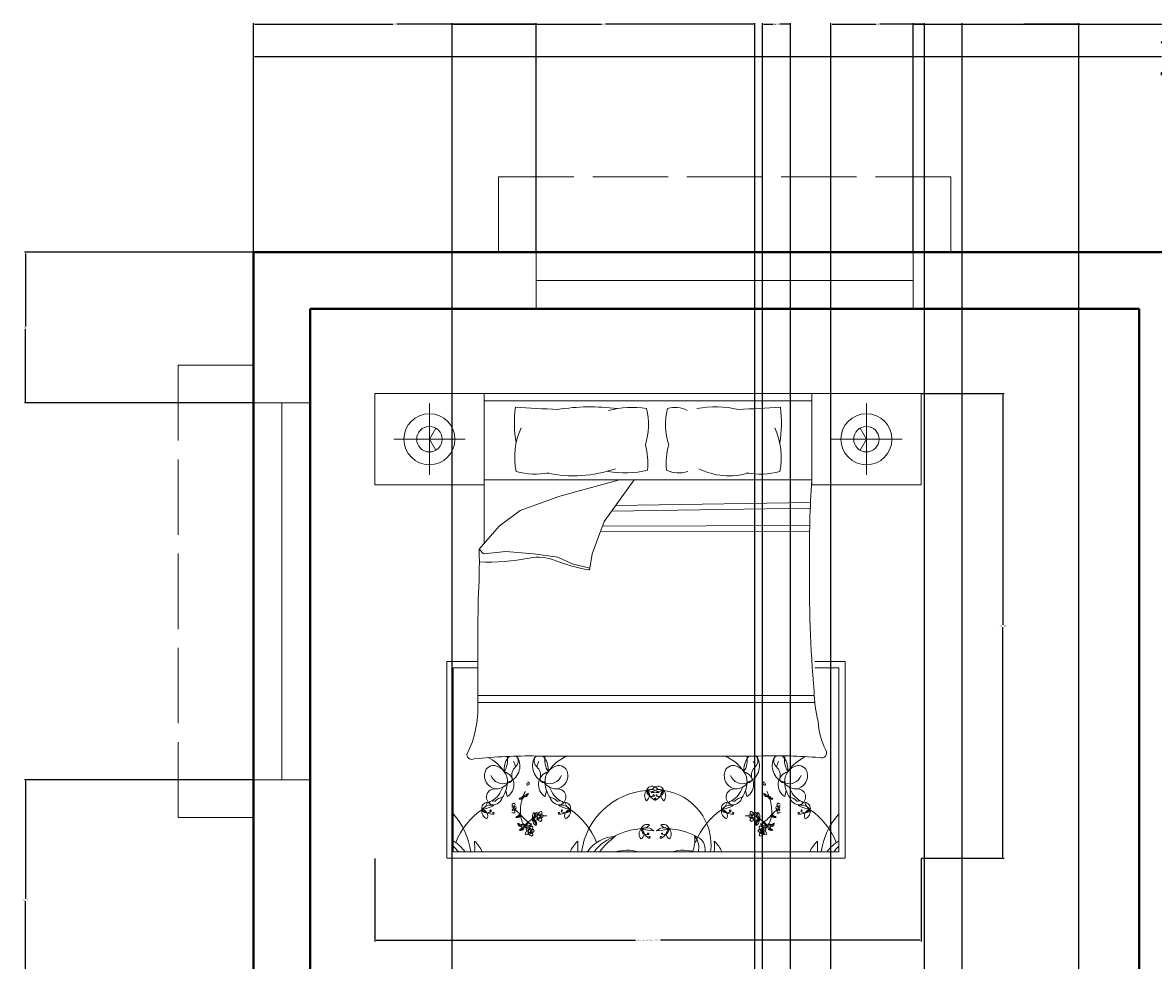
# Model space of a CAD drawing. Units: inches. Extents: x -22 to 362, y -469 to 42.
# Tile 5 of 6: x -22 to 158, y -107 to 42. Entities that reach past the tile are written whole.
import ezdxf

# ---------------------------------------------------------------- set-up
doc = ezdxf.new("R2010")
doc.units = ezdxf.units.IN
doc.header["$MEASUREMENT"] = 0
doc.linetypes.add('ACAD_ISO02W100', pattern=[15, 12, -3])
for name, color, linetype, lineweight in [('A-ANNO-DIMS', 2, 'Continuous', 18), ('A-FURN', 8, 'Continuous', 18), ('A-GLAZ', 4, 'Continuous', 20), ('A-ROOF-OVHD', 8, 'ACAD_ISO02W100', 18), ('A-WALL', 7, 'Continuous', 40)]:
    doc.layers.add(name, color=color, linetype=linetype, lineweight=lineweight)
doc.styles.get("Standard").update_dxf_attribs({"font": 'arial.ttf'})
doc.dimstyles.get("Standard").update_dxf_attribs({"dimtxt": 0.18, "dimasz": 0.18, "dimexe": 0.18, "dimexo": 0.0625, "dimgap": 0.09, "dimtad": 0, "dimtih": 1, "dimtoh": 1, "dimdec": 0, "dimzin": 0, "dimdsep": 46, "dimlunit": 3, "dimtxsty": 'Standard', "dimcen": 0.09, "dimadec": 0, "dimazin": 0, "dimtfac": 1, "dimtdec": 0, "dimtofl": 0, "dimtmove": 0, "dimatfit": 3, "dimfxl": 1, "dimtolj": 1, "dimtzin": 0, "dimarcsym": 0})

# ---------------------------------------------------------------- blocks, each defined once
blk = doc.blocks.new('*D5')
at = {"layer": 'A-ANNO-DIMS', "color": 0, "lineweight": -2, "transparency": 16777216}
for p, q in [((15.01, 5.76), (15.01, 37.04)), ((15.19, 36.86), (159.53, 36.86)), ((314.33, 36.86), (169.99, 36.86)), ((314.51, 5.76), (314.51, 37.04))]:
    blk.add_line(p, q, dxfattribs=at)
at = {"layer": 'A-ANNO-DIMS', "color": 0, "transparency": 16777216}
for points in [[(15.19, 36.89), (15.19, 36.83), (15.01, 36.86)], [(314.33, 36.89), (314.33, 36.83), (314.51, 36.86)]]:
    blk.add_solid(points, dxfattribs=at)
at = {"layer": 'Defpoints', "color": 0, "transparency": 16777216}
for p in [(314.51, 36.86), (15.01, 5.69), (314.51, 5.69)]:
    blk.add_point(p, dxfattribs=at)
at = {"layer": 'A-ANNO-DIMS', "color": 0, "transparency": 16777216, "insert": (164.76, 36.86), "char_height": 6, "attachment_point": 5}
blk.add_mtext("\\A1;25'", dxfattribs=at)
blk = doc.blocks.new('WIN-60-WALL9')
for p, q in [((0, 9), (60, 9)), ((0, 0), (0, 9)), ((60, 9), (60, 0)), ((0, 4.5), (60, 4.5)), ((60, 0), (0, 0))]:
    blk.add_line(p, q)
blk = doc.blocks.new('WINDOW-SHADE-72')
for p, q in [((12, 72), (0, 72)), ((12, 0), (12, 72)), ((0, 0), (12, 0))]:
    blk.add_line(p, q)
blk = doc.blocks.new('BED-DOUBLE-WITH-NIGHTSTANDS')
for p, q in [((0, 73.94), (86.94, 73.94)), ((17.39, 73.94), (17.39, 50.07)), ((8.69, 61.01), (8.69, 72.37)), ((69.55, 72.82), (17.39, 72.82)), ((78.25, 61.01), (78.25, 72.37)), ((14.37, 66.69), (3.01, 66.69)), ((72.57, 66.69), (83.93, 66.69)), ((17.39, 60.2), (69.55, 60.2)), ((29.46, 57.61), (38.94, 60.2)), ((41.27, 60.2), (36.51, 53.57)), ((23.13, 55.33), (29.46, 57.61)), ((69.32, 56.59), (38.37, 56.15)), ((19.78, 52.86), (23.13, 55.33)), ((69.29, 55.69), (37.72, 55.25)), ((16.61, 49.17), (19.78, 52.86)), ((36.51, 53.57), (34.57, 48.46)), ((69.24, 52.96), (36.23, 52.83)), ((69.24, 52.06), (35.89, 51.93)), ((17.31, 48.46), (16.61, 49.17)), ((20.84, 48.81), (17.31, 48.46)), ((25.24, 48.46), (20.84, 48.81)), ((29.11, 47.94), (25.24, 48.46)), ((31.4, 46.88), (29.11, 47.94)), ((34.22, 46.18), (31.4, 46.88)), ((34.57, 48.46), (34.22, 46.18)), ((11.48, 31.32), (16.39, 31.32)), ((11.48, 0), (11.48, 31.32)), ((70.04, 31.32), (74.86, 31.32)), ((74.86, 31.32), (74.86, 0)), ((16.39, 30.31), (12.48, 30.31)), ((12.48, 30.31), (12.48, 1.01)), ((73.85, 30.31), (70.02, 30.31)), ((73.85, 1.01), (73.85, 30.31)), ((69.95, 25.9), (16.39, 25.9)), ((70.03, 24.81), (16.39, 24.81)), ((61.12, 16.27), (25.82, 16.27)), ((21.05, 9.82), (20.86, 10.8)), ((27.13, 9.82), (27.32, 10.8)), ((59.21, 9.82), (59.02, 10.8)), ((65.28, 9.82), (65.48, 10.8)), ((74.86, 0), (11.48, 0)), ((12.48, 1.01), (73.85, 1.01))]:
    blk.add_line(p, q)
for points in [[(17.39, 59.45), (0, 59.45), (0, 73.94)], [(69.55, 73.94), (69.55, 59.45), (86.94, 59.45), (86.94, 73.94)], [(8.69, 66.69), (9.71, 68.45)], [(78.25, 66.69), (77.23, 68.45)], [(8.69, 66.69), (9.71, 64.94)], [(78.25, 66.69), (77.23, 64.94)]]:
    blk.add_lwpolyline(points)
for points in [[(22.38, 71.77, 0.074897), (22.49, 66.09, -0.472817)], [(43.06, 65.77, 0.14099), (43.24, 71.57, 0.235245)], [(46.78, 65.77, -0.14099), (46.6, 71.57, -0.235245)], [(64.56, 71.77, -0.074897), (64.45, 66.09, 0.472817)], [(16.43, 41.21, 0.001242), (16.39, 24.71, -0.127202), (14.64, 16.49)], [(69.92, 26.58, 0.056112), (70.55, 21.8, 0.095341), (71.78, 17.19)]]:
    blk.add_lwpolyline(points, format="xyb")
for centre, radius in [((8.69, 66.69), 4.06), ((78.25, 66.69), 4.06), ((8.69, 66.69), 2.03), ((78.25, 66.69), 2.03), ((26.07, 6.67), 0.221), ((60.26, 6.67), 0.221), ((24.62, 4.34), 0.221), ((61.71, 4.34), 0.221)]:
    blk.add_circle(centre, radius)
for centre, radius, start, end in [((70.3, 899.16), 828.77, 266.68521, 267.14978), ((34.29, 40.31), 31.53, 82.2196, 99.497), ((40.95, 56.24), 15.49, 81.5249, 103.96), ((47.79, 67.44), 4.3, 63.3437, 106.1026), ((54.24, 56.56), 15.28, 76.3427, 101.1841), ((16.64, 899.16), 828.77, 272.85022, 273.31479), ((33.46, 63.81), 11.21, 155.1316, 191.7583), ((53.48, 63.81), 11.21, 348.2417, 24.8684), ((32.81, 62.87), 10.65, 354.0129, 15.8293), ((57.02, 62.87), 10.65, 164.1707, 185.9871), ((25.48, 72.79), 11.65, 255.1039, 281.0369), ((31.62, 81.07), 20.21, 258.0397, 289.2615), ((39.8, 76.66), 15.33, 259.8617, 283.6238), ((48.38, 65.93), 4.61, 245.0183, 288.5407), ((56.43, 71.93), 11.07, 243.8761, 286.1746), ((61.46, 72.79), 11.65, 258.9631, 284.8961), ((225.41, 49.57), 156.22, 176.1, 180.9282), ((-63.11, 47.01), 79.74, 355.8294, 1.553), ((18.1, 79.95), 32.81, 267.4519, 281.3392), ((25.94, 40.84), 7.08, 66.2616, 101.3392), ((40.26, 79.03), 33.72, 250.1194, 259.3383), ((272.96, 43.89), 203.78, 179.1145, 184.8735), ((34.02, 46.1), 0.21, 268.8623, 19.7536), ((15.44, 16.54), 0.802, 183.98, 297.3412), ((24.78, -74.23), 90.51, 89.3433, 95.6887), ((17.52, 15.63), 3.6, 328.8218, 9.1554), ((21.98, 15.31), 1.05, 120.0293, 142.325), ((21.98, 15.31), 1.05, 44.4517, 63.558), ((26.2, 15.31), 1.05, 113.229, 135.5483), ((26.2, 15.31), 1.05, 37.675, 66.7144), ((30.66, 15.63), 3.6, 169.7133, 211.1782), ((33.07, 10.15), 6.58, 111.4941, 146.3329), ((53.26, 10.15), 6.58, 33.6671, 68.5059), ((55.68, 15.63), 3.6, 328.8218, 10.2867), ((60.14, 15.31), 1.05, 113.2856, 142.325), ((60.14, 15.31), 1.05, 44.4517, 66.7144), ((63.78, -68.29), 84.6, 85.2402, 91.8035), ((64.35, 15.31), 1.05, 106.6343, 135.5483), ((64.35, 15.31), 1.05, 37.675, 72.5814), ((68.82, 15.63), 3.6, 169.249, 211.1782), ((71.12, 16.75), 0.792, 246.5219, 33.8264), ((18.94, 13.31), 1.47, 84.4856, 181.0538), ((15.1, 10.15), 6.58, 33.6671, 63.2997), ((18.49, 12.22), 2.61, 355.2933, 76.921), ((23.92, 14.06), 3.35, 145.785, 184.7304), ((20.31, 14.69), 2.77, 289.2822, 29.1751), ((23.58, 13.21), 1.78, 131.5653, 195.1471), ((19.89, 14.19), 2.5, 7.436, 29.9149), ((21.54, 15.52), 1.3, 311.5653, 23.8354), ((27.87, 14.69), 2.77, 150.8249, 250.7178), ((26.64, 15.52), 1.3, 156.1646, 228.4347), ((24.59, 13.21), 1.78, 344.8529, 48.4347), ((28.29, 14.19), 2.5, 150.0851, 172.564), ((24.25, 14.06), 3.35, 355.2696, 34.215), ((29.69, 12.22), 2.61, 103.079, 184.7067), ((29.24, 13.31), 1.47, 358.9462, 95.5144), ((57.09, 13.31), 1.47, 84.4856, 181.0538), ((56.64, 12.22), 2.61, 355.2933, 76.921), ((62.08, 14.06), 3.35, 145.785, 184.7304), ((58.46, 14.69), 2.77, 289.2822, 29.1751), ((61.74, 13.21), 1.78, 131.5653, 195.1471), ((58.05, 14.19), 2.5, 7.436, 29.9149), ((59.69, 15.52), 1.3, 311.5653, 23.8354), ((66.03, 14.69), 2.77, 150.8249, 250.7178), ((64.8, 15.52), 1.3, 156.1646, 228.4347), ((62.75, 13.21), 1.78, 344.8529, 48.4347), ((66.44, 14.19), 2.5, 150.0851, 172.564), ((62.41, 14.06), 3.35, 355.2696, 34.215), ((67.85, 12.22), 2.61, 103.079, 184.7067), ((71.23, 10.15), 6.58, 113.6453, 146.3329), ((67.4, 13.31), 1.47, 358.9462, 95.5144), ((19.54, 13.1), 2.08, 174.9449, 262.8857), ((20.36, 13.89), 2.02, 201.5819, 291.4221), ((19.97, 11.7), 2.16, 299.9085, 73.1337), ((21.34, 12.6), 0.54, 257.3041, 15.1471), ((28.2, 11.7), 2.16, 106.8663, 240.0915), ((26.84, 12.6), 0.54, 164.8529, 282.6959), ((27.82, 13.89), 2.02, 248.5779, 338.4181), ((28.64, 13.1), 2.08, 277.1143, 5.0551), ((57.7, 13.1), 2.08, 174.9449, 262.8857), ((58.51, 13.89), 2.02, 201.5819, 291.4221), ((58.13, 11.7), 2.16, 299.9085, 73.1337), ((59.5, 12.6), 0.54, 257.3041, 15.1471), ((66.36, 11.7), 2.16, 106.8663, 240.0915), ((64.99, 12.6), 0.54, 164.8529, 282.6959), ((65.98, 13.89), 2.02, 248.5779, 338.4181), ((66.79, 13.1), 2.08, 277.1143, 5.0551), ((19.06, 9.75), 1.3, 80.264, 250.8688), ((16.47, 12.62), 4.1, 301.2614, 341.7045), ((19.18, 13.56), 2.53, 272.3591, 324.0401), ((16.44, 12.29), 4.67, 326.2883, 356.5076), ((23.92, 14.06), 3.35, 212.7011, 216.3445), ((24.34, 11.79), 0.168, 102.7051, 280.4384), ((24.32, 11.89), 0.272, 280.4384, 100.4136), ((24.25, 14.06), 3.35, 323.6555, 327.2989), ((29, 13.56), 2.53, 215.9599, 267.6409), ((31.74, 12.29), 4.67, 183.4924, 213.7117), ((31.7, 12.62), 4.1, 198.2955, 238.7386), ((29.12, 9.75), 1.3, 289.1312, 99.736), ((44.17, 10.53), 0.941, 63.0274, 163.8037), ((43.21, 12.73), 1.94, 271.4585, 315.3727), ((44, 9.16), 1.79, 45.5411, 114.3101), ((45.23, 9.16), 1.79, 65.6899, 134.4589), ((45.07, 10.53), 0.941, 16.1963, 116.9726), ((46.02, 12.73), 1.94, 224.6273, 268.5415), ((57.22, 9.75), 1.3, 80.264, 250.8688), ((54.63, 12.62), 4.1, 301.2614, 341.7045), ((57.34, 13.56), 2.53, 272.3591, 324.0401), ((54.59, 12.29), 4.67, 326.2883, 356.5076), ((62.08, 14.06), 3.35, 212.7011, 216.3445), ((62.01, 11.89), 0.272, 79.5864, 259.5616), ((62, 11.79), 0.168, 259.5616, 77.2949), ((62.41, 14.06), 3.35, 323.6555, 327.2989), ((67.16, 13.56), 2.53, 215.9599, 267.6409), ((69.9, 12.29), 4.67, 183.4924, 213.7117), ((69.86, 12.62), 4.1, 198.2955, 238.7386), ((67.27, 9.75), 1.3, 289.1312, 99.736), ((18.79, 8.34), 0.8, 63.9755, 143.2681), ((18.75, 10.14), 1.63, 265.969, 344.3045), ((20.5, 7.98), 1.74, 96.1662, 141.5825), ((23.38, 9.2), 0.456, 101.3256, 154.4621), ((22.72, 10.74), 1.37, 280.2588, 300.656), ((23.04, 11.84), 2.45, 268.3264, 277.1302), ((30.36, 7.41), 7.2, 163.5842, 183.8277), ((22.42, 10.74), 1.4, 308.2101, 316.3071), ((23.28, 9.82), 0.417, 278.3432, 4.2869), ((23.05, 10.19), 0.729, 300.656, 332.6341), ((23.6, 9.71), 0.177, 55.7657, 157.4417), ((30.36, 7.41), 7.2, 153.0032, 159.8941), ((23.87, 9.87), 0.177, 84.3784, 186.0543), ((23.71, 10.58), 0.729, 269.1859, 301.164), ((23.92, 10.21), 0.417, 237.5332, 323.4768), ((23.52, 11.4), 1.4, 285.5129, 293.6099), ((23.37, 11.14), 1.37, 301.164, 321.5612), ((24.43, 9.82), 0.456, 87.3579, 140.4944), ((22.26, 11.38), 2.45, 324.6898, 333.4936), ((27.67, 7.98), 1.74, 38.4175, 83.8338), ((29.43, 10.14), 1.63, 195.6955, 274.031), ((29.38, 8.34), 0.8, 36.7319, 116.0245), ((44.15, -0.52), 11.35, 94.4623, 172.255), ((44.2, 9.95), 1.26, 137.7873, 219.1145), ((42.77, 9.99), 0.948, 298.5391, 58.3627), ((45.64, 18.38), 7.94, 252.593, 267.2582), ((44.19, 10.76), 0.929, 177.7585, 283.852), ((45.98, 11.73), 2.87, 198.9159, 238.011), ((43.59, 18.38), 7.94, 272.7418, 287.407), ((44.38, 9.98), 0.123, 283.852, 219.9245), ((44.53, 9.41), 0.141, 238.011, 71.5592), ((44.56, 9.48), 0.0685, 71.5592, 188.0167), ((44.7, 9.41), 0.141, 108.4408, 301.989), ((44.68, 9.48), 0.0685, 351.9833, 108.4408), ((44.84, 10.03), 0.074, 320.1909, 256.0209), ((43.25, 11.73), 2.87, 301.989, 341.0841), ((45.04, 10.76), 0.929, 256.148, 2.2415), ((46.47, 9.99), 0.948, 121.6373, 241.4609), ((45.04, 9.95), 1.26, 320.8855, 42.2127), ((44.72, 2.1), 8.79, 352.8636, 81.8197), ((56.95, 8.34), 0.8, 63.9755, 143.2681), ((56.91, 10.14), 1.63, 265.969, 344.3045), ((58.66, 7.98), 1.74, 96.1662, 141.5825), ((62.96, 11.14), 1.37, 218.4388, 238.836), ((61.9, 9.82), 0.456, 39.5056, 92.6421), ((64.08, 11.38), 2.45, 206.5064, 215.3102), ((62.41, 10.21), 0.417, 216.5232, 302.4668), ((62.63, 10.58), 0.729, 238.836, 270.8141), ((62.82, 11.4), 1.4, 246.3901, 254.4871), ((55.97, 7.41), 7.2, 20.1059, 26.9968), ((62.46, 9.87), 0.177, 353.9457, 95.6216), ((62.74, 9.71), 0.177, 22.5583, 124.2343), ((63.05, 9.82), 0.417, 175.7131, 261.6568), ((63.28, 10.19), 0.729, 207.3659, 239.344), ((55.97, 7.41), 7.2, 356.1723, 16.4158), ((63.91, 10.74), 1.4, 223.6929, 231.7899), ((63.61, 10.74), 1.37, 239.344, 259.7412), ((63.3, 11.84), 2.45, 262.8698, 271.6736), ((62.96, 9.2), 0.456, 25.5379, 78.6744), ((67.59, 10.14), 1.63, 195.6955, 274.031), ((65.83, 7.98), 1.74, 38.4175, 83.8338), ((67.54, 8.34), 0.8, 36.7319, 116.0245), ((23.45, -1.64), 11.35, 124.3865, 158.5908), ((18.27, 7.46), 1.26, 167.7115, 249.0387), ((17.96, 7.95), 0.941, 92.9516, 193.728), ((16.03, 9.38), 1.94, 301.3827, 345.2969), ((18.5, 6.68), 1.79, 75.4653, 144.2343), ((15.32, 15.48), 7.94, 282.5173, 297.1824), ((17.01, 6.78), 0.948, 328.4633, 88.2869), ((18.93, 9.89), 2.87, 228.8402, 267.9352), ((17.86, 8.16), 0.929, 207.6827, 313.7762), ((18.42, 7.57), 0.123, 313.7762, 249.7183), ((18.82, 7.23), 0.0685, 101.4834, 217.9409), ((18.83, 7.16), 0.141, 267.9352, 101.4834), ((22.09, 8.33), 0.369, 101.5637, 142.6358), ((21.78, 7.99), 0.221, 273.2768, 86.7232), ((22.08, 7.58), 0.366, 217.7621, 259.0403), ((22.04, 8.2), 0.211, 91.1081, 181.8675), ((22.48, 8.06), 0.672, 203.4276, 227.6104), ((22.26, 7.77), 0.458, 80.3487, 133.6538), ((22.18, 8.15), 0.362, 229.7889, 317.6792), ((21.79, 8.62), 0.532, 288.7263, 352.5032), ((21.77, 7.38), 0.515, 355.053, 68.3618), ((22.18, 7.3), 0.725, 83.0852, 105.7171), ((22.15, 8.59), 0.171, 345.2356, 144.9248), ((22.12, 7.35), 0.17, 232.4737, 355.053), ((17.16, 1.28), 8.25, 43.1541, 52.0459), ((22.31, 8.03), 0.191, 317.6792, 80.3487), ((24.38, 7), 1.01, 304.5369, 16.3699), ((25.78, 6.72), 0.714, 127.3105, 187.9252), ((24.8, 6.8), 0.733, 355.0106, 41.658), ((25.83, 6.98), 0.302, 126.1046, 271.4281), ((25.8, 7.06), 0.217, 353.7526, 131.7054), ((26.38, 7.01), 0.369, 101.5637, 176.365), ((26.08, 7.3), 0.532, 288.7263, 352.5032), ((26.45, 7.28), 0.171, 345.2356, 144.9248), ((29.34, 7.16), 0.141, 78.5166, 272.0648), ((29.68, 6.68), 1.79, 35.7657, 104.5347), ((32.86, 15.48), 7.94, 242.8176, 257.4827), ((29.24, 9.89), 2.87, 272.0648, 311.1598), ((29.36, 7.23), 0.0685, 322.0591, 78.5166), ((30.31, 8.16), 0.929, 226.2238, 332.3173), ((29.77, 7.62), 0.074, 290.2667, 226.2271), ((31.16, 6.78), 0.948, 91.7131, 211.5367), ((30.22, 7.95), 0.941, 346.272, 87.0484), ((32.14, 9.38), 1.94, 194.7031, 238.6173), ((29.9, 7.46), 1.26, 290.9613, 12.2885), ((24.72, -1.64), 11.35, 21.4092, 55.6135), ((61.61, -1.64), 11.35, 124.3865, 158.5908), ((56.11, 7.95), 0.941, 92.9516, 193.728), ((56.43, 7.46), 1.26, 167.7115, 249.0387), ((54.19, 9.38), 1.94, 301.3827, 345.2969), ((56.66, 6.68), 1.79, 75.4653, 144.2343), ((53.48, 15.48), 7.94, 282.5173, 297.1824), ((56.02, 8.16), 0.929, 207.6827, 313.7762), ((57.09, 9.89), 2.87, 228.8402, 267.9352), ((55.17, 6.78), 0.948, 328.4633, 88.2869), ((56.58, 7.57), 0.123, 313.7762, 249.7183), ((56.98, 7.23), 0.0685, 101.4834, 217.9409), ((56.99, 7.16), 0.141, 267.9352, 101.4834), ((59.89, 7.28), 0.171, 35.0752, 194.7644), ((60.25, 7.3), 0.532, 187.4968, 251.2737), ((59.95, 7.01), 0.369, 3.635, 78.4363), ((60.54, 7.06), 0.217, 48.2946, 186.2474), ((60.51, 6.98), 0.302, 268.5719, 53.8954), ((61.54, 6.8), 0.733, 138.342, 184.9894), ((61.96, 7), 1.01, 163.6301, 235.4631), ((60.55, 6.72), 0.714, 352.0748, 52.6895), ((69.18, 1.28), 8.25, 127.9541, 136.8459), ((64.03, 8.03), 0.191, 99.6513, 222.3208), ((64.15, 8.15), 0.362, 222.3208, 310.2111), ((64.07, 7.77), 0.458, 46.3462, 99.6513), ((64.18, 8.59), 0.171, 35.0752, 194.7644), ((64.54, 8.62), 0.532, 187.4968, 251.2737), ((64.56, 7.38), 0.515, 111.6382, 184.947), ((64.22, 7.35), 0.17, 184.947, 307.5263), ((64.16, 7.3), 0.725, 74.2829, 96.9148), ((64.29, 8.2), 0.211, 358.1325, 88.8919), ((63.86, 8.06), 0.672, 312.3896, 336.5724), ((64.25, 8.33), 0.369, 37.3642, 78.4363), ((64.25, 7.58), 0.366, 280.9597, 322.2379), ((64.55, 7.99), 0.221, 93.2768, 266.7232), ((67.5, 7.16), 0.141, 78.5166, 272.0648), ((67.84, 6.68), 1.79, 35.7657, 104.5347), ((71.01, 15.48), 7.94, 242.8176, 257.4827), ((67.4, 9.89), 2.87, 272.0648, 311.1598), ((67.51, 7.23), 0.0685, 322.0591, 78.5166), ((68.47, 8.16), 0.929, 226.2238, 332.3173), ((67.93, 7.62), 0.074, 290.2667, 226.2271), ((69.32, 6.78), 0.948, 91.7131, 211.5367), ((70.3, 9.38), 1.94, 194.7031, 238.6173), ((68.38, 7.95), 0.941, 346.272, 87.0484), ((68.06, 7.46), 1.26, 290.9613, 12.2885), ((62.88, -1.64), 11.35, 21.4092, 55.6135), ((4.03, -0.52), 11.35, 7.745, 41.8856), ((22.86, 6.27), 0.456, 101.3256, 154.4621), ((22.2, 7.82), 1.37, 280.2588, 300.656), ((22.52, 8.92), 2.45, 268.3264, 277.1302), ((21.91, 7.82), 1.4, 308.2101, 316.3071), ((23.01, 5.47), 0.247, 146.8636, 236.9021), ((26.5, 10.92), 6.47, 235.1882, 238.8844), ((23.44, 5.83), 0.669, 199.4799, 267.6828), ((22.76, 6.9), 0.417, 278.3432, 4.2869), ((22.53, 7.26), 0.729, 300.656, 332.6341), ((23.08, 6.78), 0.177, 55.7657, 157.4417), ((23.29, 5.6), 0.256, 238.8844, 314.2646), ((26.78, 7.23), 3.61, 184.756, 209.2041), ((31.97, 14.91), 11.88, 222.2412, 232.1744), ((23.6, 5.27), 0.193, 311.8703, 134.2646), ((24.16, 6.15), 1.01, 247.2305, 319.0635), ((27.15, 2.43), 4.33, 120.544, 139.818), ((24.68, 4.82), 0.714, 70.0041, 130.6188), ((24.22, 5.69), 0.733, 297.7043, 344.3516), ((24.92, 6.78), 0.613, 272.8499, 356.1226), ((24.48, 6.54), 0.594, 321.7607, 7.9252), ((24.61, 5.68), 0.594, 8.7227, 54.8872), ((24.64, 5.21), 1.01, 0.278, 72.111), ((25.09, 5.58), 0.613, 20.5253, 88.5375), ((25.9, 5.88), 0.714, 188.7227, 249.3375), ((25.61, 6.26), 0.219, 148.0499, 225.6268), ((27.15, 2.43), 4.33, 113.0501, 113.8477), ((26.01, 6), 0.698, 104.7558, 148.0499), ((25.62, 6.5), 0.437, 247.4086, 351.4386), ((24.99, 5.52), 0.733, 334.9899, 21.6373), ((25.75, 6.48), 0.147, 262.906, 7.132), ((25.59, 6.8), 0.305, 0.0645, 61.1507), ((25.66, 7.06), 0.348, 311.8413, 355.7877), ((26.37, 6.26), 0.366, 151.2196, 259.0403), ((26.33, 6.88), 0.211, 91.1081, 181.8675), ((26.77, 6.75), 0.672, 203.4276, 227.6104), ((26.56, 6.46), 0.458, 80.3487, 133.6538), ((26.47, 6.83), 0.362, 229.7889, 317.6792), ((26.07, 6.07), 0.515, 355.053, 68.3618), ((26.47, 5.98), 0.725, 83.0852, 105.7171), ((26.41, 6.04), 0.17, 232.4737, 355.053), ((26.6, 6.72), 0.191, 317.6792, 80.3487), ((27.15, 2.43), 4.33, 87.1071, 94.7585), ((59.19, 2.43), 4.33, 85.2415, 92.8929), ((59.73, 6.72), 0.191, 99.6513, 222.3208), ((59.86, 6.83), 0.362, 222.3208, 310.2111), ((59.78, 6.46), 0.458, 46.3462, 99.6513), ((60.27, 6.07), 0.515, 111.6382, 184.947), ((59.93, 6.04), 0.17, 184.947, 307.5263), ((59.87, 5.98), 0.725, 74.2829, 96.9148), ((60, 6.88), 0.211, 358.1325, 88.8919), ((59.56, 6.75), 0.672, 312.3896, 336.5724), ((59.96, 6.26), 0.366, 280.9597, 28.7804), ((60.71, 6.5), 0.437, 188.5614, 292.5914), ((60.67, 7.06), 0.348, 184.2123, 228.1587), ((60.74, 6.8), 0.305, 118.8493, 179.9355), ((60.59, 6.48), 0.147, 172.868, 277.094), ((60.32, 6), 0.698, 31.9501, 75.2442), ((61.35, 5.52), 0.733, 158.3627, 205.0101), ((61.24, 5.58), 0.613, 91.4625, 159.4747), ((61.69, 5.21), 1.01, 107.889, 179.722), ((60.43, 5.88), 0.714, 290.6625, 351.2773), ((61.42, 6.78), 0.613, 183.8774, 267.1501), ((59.19, 2.43), 4.33, 66.1523, 66.9499), ((60.73, 6.26), 0.219, 314.3732, 31.9501), ((61.73, 5.68), 0.594, 125.1128, 171.2773), ((61.85, 6.54), 0.594, 172.0748, 218.2393), ((59.19, 2.43), 4.33, 40.182, 59.456), ((61.65, 4.82), 0.714, 49.3812, 109.9959), ((62.17, 6.15), 1.01, 220.9365, 292.7695), ((62.11, 5.69), 0.733, 195.6484, 242.2957), ((54.36, 14.91), 11.88, 307.8256, 317.7588), ((62.73, 5.27), 0.193, 45.7354, 228.1297), ((59.56, 7.23), 3.61, 330.7959, 355.244), ((63.04, 5.6), 0.256, 225.7354, 301.1156), ((62.9, 5.83), 0.669, 272.3172, 340.5201), ((63.25, 6.78), 0.177, 22.5583, 124.2343), ((63.57, 6.9), 0.417, 175.7131, 261.6568), ((63.8, 7.26), 0.729, 207.3659, 239.344), ((59.83, 10.92), 6.47, 301.1156, 304.8118), ((64.43, 7.82), 1.4, 223.6929, 231.7899), ((64.13, 7.82), 1.37, 239.344, 259.7412), ((63.32, 5.47), 0.247, 303.0979, 33.1364), ((63.81, 8.92), 2.45, 262.8698, 271.6736), ((63.47, 6.27), 0.456, 25.5379, 78.6744), ((82.3, -0.52), 11.35, 138.1144, 172.255), ((23.36, 5.57), 0.576, 212.8155, 277.3992), ((23.03, 5.19), 0.669, 266.9701, 338.2913), ((19.5, 9.97), 6.47, 302.6784, 306.3746), ((23.2, 4.66), 0.247, 214.3538, 304.3923), ((23.23, 5.02), 0.576, 280.3057, 17.1958), ((23.18, 4.96), 0.256, 306.3746, 21.7548), ((23.6, 5.13), 0.193, 19.3605, 201.7548), ((27.23, 3.52), 3.86, 153.7819, 158.2913), ((23.83, 5.81), 0.594, 264.4544, 310.6188), ((26.78, 7.23), 3.61, 214.0033, 222.4917), ((24.27, 5.57), 0.613, 218.3208, 298.8162), ((24.16, 3.92), 0.219, 148.0499, 225.6268), ((24.57, 3.67), 0.698, 104.7558, 148.0499), ((24.17, 4.17), 0.437, 247.4086, 351.4386), ((24.38, 4.65), 0.302, 126.1046, 271.4281), ((24.35, 4.73), 0.217, 353.7526, 131.7054), ((24.3, 4.15), 0.147, 262.906, 7.132), ((24.14, 4.47), 0.305, 0.0645, 61.1507), ((24.22, 4.73), 0.348, 311.8413, 355.7877), ((24.93, 4.68), 0.369, 101.5637, 176.365), ((24.93, 3.93), 0.366, 151.2196, 259.0403), ((24.88, 4.55), 0.211, 91.1081, 181.8675), ((25.32, 4.41), 0.672, 203.4276, 227.6104), ((25.11, 4.12), 0.458, 80.3487, 133.6538), ((25.03, 4.5), 0.362, 229.7889, 317.6792), ((24.63, 4.97), 0.532, 288.7263, 352.5032), ((24.62, 3.73), 0.515, 355.053, 68.3618), ((25.02, 3.65), 0.725, 83.0852, 105.7171), ((25, 4.94), 0.171, 345.2356, 144.9248), ((24.96, 3.7), 0.17, 232.4737, 355.053), ((25.15, 4.39), 0.191, 317.6792, 80.3487), ((43.28, -6.6), 11.35, 94.4623, 117.4146), ((43.33, 3.87), 1.26, 137.7873, 219.1145), ((41.9, 3.91), 0.948, 298.5391, 58.3627), ((43.3, 4.45), 0.941, 63.0274, 163.8037), ((42.34, 6.65), 1.94, 271.4585, 315.3727), ((43.13, 3.08), 1.79, 45.5411, 114.3101), ((45.11, 5.65), 2.87, 198.9159, 238.011), ((44.77, 12.29), 7.94, 252.593, 267.2582), ((43.32, 4.68), 0.929, 177.7585, 283.852), ((43.51, 3.9), 0.123, 283.852, 219.9245), ((46.1, 3.08), 1.79, 65.6899, 134.4589), ((44.46, 12.29), 7.94, 272.7418, 287.407), ((45.93, 4.45), 0.941, 16.1963, 116.9726), ((46.89, 6.65), 1.94, 224.6273, 268.5415), ((45.71, 3.94), 0.074, 320.1909, 256.0209), ((44.12, 5.65), 2.87, 301.989, 341.0841), ((45.91, 4.68), 0.929, 256.148, 2.2415), ((47.34, 3.91), 0.948, 121.6373, 241.4609), ((45.91, 3.87), 1.26, 320.8855, 42.2127), ((45.95, -6.6), 11.35, 62.5854, 85.5377), ((61.18, 4.39), 0.191, 99.6513, 222.3208), ((61.31, 4.5), 0.362, 222.3208, 310.2111), ((61.23, 4.12), 0.458, 46.3462, 99.6513), ((61.34, 4.94), 0.171, 35.0752, 194.7644), ((61.7, 4.97), 0.532, 187.4968, 251.2737), ((61.72, 3.73), 0.515, 111.6382, 184.947), ((61.37, 3.7), 0.17, 184.947, 307.5263), ((61.31, 3.65), 0.725, 74.2829, 96.9148), ((61.45, 4.55), 0.211, 358.1325, 88.8919), ((61.01, 4.41), 0.672, 312.3896, 336.5724), ((61.4, 4.68), 0.369, 3.635, 78.4363), ((61.41, 3.93), 0.366, 280.9597, 28.7804), ((62.16, 4.17), 0.437, 188.5614, 292.5914), ((62.07, 5.57), 0.613, 241.1838, 321.6792), ((61.99, 4.73), 0.217, 48.2946, 186.2474), ((62.12, 4.73), 0.348, 184.2123, 228.1587), ((62.19, 4.47), 0.305, 118.8493, 179.9355), ((62.04, 4.15), 0.147, 172.868, 277.094), ((61.95, 4.65), 0.302, 268.5719, 53.8954), ((61.77, 3.67), 0.698, 31.9501, 75.2442), ((62.5, 5.81), 0.594, 229.3812, 275.5456), ((59.56, 7.23), 3.61, 317.5083, 325.9967), ((62.17, 3.92), 0.219, 314.3732, 31.9501), ((63.1, 5.02), 0.576, 162.8042, 259.6943), ((62.73, 5.13), 0.193, 338.2452, 160.6395), ((59.1, 3.52), 3.86, 21.7087, 26.2181), ((63.31, 5.19), 0.669, 201.7087, 273.0299), ((63.15, 4.96), 0.256, 158.2452, 233.6254), ((62.97, 5.57), 0.576, 262.6008, 327.1845), ((66.83, 9.97), 6.47, 233.6254, 237.3216), ((63.14, 4.66), 0.247, 235.6077, 325.6462), ((9.73, -2.04), 5.53, 33.4617, 60.1116), ((7.74, -3.07), 6.89, 36.3036, 46.4814), ((12.82, -0.76), 4.62, 22.5547, 48.9546), ((0.18, 1.72), 15.71, 357.4081, 3.6519), ((35.35, -0.76), 4.62, 131.0454, 157.4453), ((48, 1.72), 15.71, 176.3481, 182.5919), ((38.45, -2.04), 5.53, 91.272, 146.5383), ((40.44, -3.07), 6.89, 107.8504, 143.6964), ((44.06, -5.01), 10.25, 124.0123, 144.053), ((43.66, 3.33), 0.141, 238.011, 71.5592), ((43.69, 3.4), 0.0685, 71.5592, 188.0167), ((45.57, 3.33), 0.141, 108.4408, 301.989), ((45.55, 3.4), 0.0685, 351.9833, 108.4408), ((45.85, 2.9), 5.08, 338.117, 6.6195), ((50.52, 1.49), 2.04, 346.3898, 79.0739), ((48.99, 1.77), 2.58, 342.8609, 41.9049), ((38.34, 1.72), 15.71, 357.4081, 3.6519), ((50.98, -0.76), 4.62, 22.5547, 48.9546), ((73.51, -0.76), 4.62, 131.0454, 157.4453), ((86.15, 1.72), 15.71, 176.3481, 182.5919), ((76.61, -2.04), 5.53, 119.8884, 146.5383), ((78.6, -3.07), 6.89, 133.5186, 143.6964), ((40.1, -4.96), 6.24, 73.5431, 107.0202), ((42.58, -8.18), 9.23, 94.3787, 95.6357), ((47.44, -14.5), 16.5, 109.7217, 109.9028), ((49.13, -4.96), 6.24, 72.9798, 106.4569), ((46.66, -8.18), 9.23, 84.3643, 85.6213), ((41.79, -14.5), 16.5, 70.0972, 70.2783)]:
    blk.add_arc(centre, radius, start, end)
blk = doc.blocks.new('*D22')
at = {"layer": 'A-ANNO-DIMS', "color": 0, "lineweight": -2, "transparency": 16777216}
for p, q in [((34.33, -90.8), (34.33, -103.96)), ((121.27, -90.8), (121.27, -103.96)), ((34.51, -103.78), (75.82, -103.78)), ((121.09, -103.78), (79.78, -103.78))]:
    blk.add_line(p, q, dxfattribs=at)
at = {"layer": 'A-ANNO-DIMS', "color": 0, "transparency": 16777216}
for points in [[(34.51, -103.75), (34.51, -103.81), (34.33, -103.78)], [(121.09, -103.75), (121.09, -103.81), (121.27, -103.78)]]:
    blk.add_solid(points, dxfattribs=at)
at = {"layer": 'Defpoints', "color": 0, "transparency": 16777216}
for p in [(34.33, -90.74), (121.27, -90.74), (121.27, -103.78)]:
    blk.add_point(p, dxfattribs=at)
at = {"layer": 'A-ANNO-DIMS', "color": 0, "transparency": 16777216, "insert": (77.8, -103.78), "char_height": 0.18, "attachment_point": 5}
blk.add_mtext('\\A1;BED & NIGHTSTANDS 7\'-3" TYP.', dxfattribs=at)
blk = doc.blocks.new('*D23')
at = {"layer": 'A-ANNO-DIMS', "color": 0, "lineweight": -2, "transparency": 16777216}
for p, q in [((121.33, -16.8), (134.49, -16.8)), ((134.31, -16.98), (134.31, -53.59)), ((134.31, -90.56), (134.31, -53.95)), ((121.33, -90.74), (134.49, -90.74))]:
    blk.add_line(p, q, dxfattribs=at)
at = {"layer": 'A-ANNO-DIMS', "color": 0, "transparency": 16777216}
for points in [[(134.28, -16.98), (134.34, -16.98), (134.31, -16.8)], [(134.28, -90.56), (134.34, -90.56), (134.31, -90.74)]]:
    blk.add_solid(points, dxfattribs=at)
at = {"layer": 'Defpoints', "color": 0, "transparency": 16777216}
for p in [(121.27, -16.8), (134.31, -16.8), (121.27, -90.74)]:
    blk.add_point(p, dxfattribs=at)
at = {"layer": 'A-ANNO-DIMS', "color": 0, "transparency": 16777216, "insert": (134.31, -53.77), "char_height": 0.18, "attachment_point": 5}
blk.add_mtext('\\A1;6\'-2" TYP.', dxfattribs=at)
blk = doc.blocks.new('*D32')
at = {"layer": 'A-ANNO-DIMS', "color": 0, "lineweight": -2, "transparency": 16777216}
for p, q in [((15.01, 5.76), (15.01, 42.15)), ((15.19, 41.97), (37.18, 41.97)), ((59.83, 41.97), (37.84, 41.97)), ((60.01, 5.76), (60.01, 42.15))]:
    blk.add_line(p, q, dxfattribs=at)
at = {"layer": 'A-ANNO-DIMS', "color": 0, "transparency": 16777216}
for points in [[(15.19, 42), (15.19, 41.94), (15.01, 41.97)], [(59.83, 42), (59.83, 41.94), (60.01, 41.97)]]:
    blk.add_solid(points, dxfattribs=at)
at = {"layer": 'Defpoints', "color": 0, "transparency": 16777216}
for p in [(60.01, 41.97), (15.01, 5.69), (60.01, 5.69)]:
    blk.add_point(p, dxfattribs=at)
at = {"layer": 'A-ANNO-DIMS', "color": 0, "transparency": 16777216, "insert": (37.51, 41.97), "char_height": 0.18, "attachment_point": 5}
blk.add_mtext('\\A1;3\'-9"', dxfattribs=at)
blk = doc.blocks.new('*D33')
at = {"layer": 'A-ANNO-DIMS', "color": 0, "lineweight": -2, "transparency": 16777216}
for p, q in [((120.01, 5.76), (120.01, 42.15)), ((120.19, 41.97), (161.11, 41.97)), ((202.83, 41.97), (161.91, 41.97)), ((203.01, 5.76), (203.01, 42.15))]:
    blk.add_line(p, q, dxfattribs=at)
at = {"layer": 'A-ANNO-DIMS', "color": 0, "transparency": 16777216}
for points in [[(120.19, 42), (120.19, 41.94), (120.01, 41.97)], [(202.83, 42), (202.83, 41.94), (203.01, 41.97)]]:
    blk.add_solid(points, dxfattribs=at)
at = {"layer": 'Defpoints', "color": 0, "transparency": 16777216}
for p in [(203.01, 41.97), (120.01, 5.69), (203.01, 5.69)]:
    blk.add_point(p, dxfattribs=at)
at = {"layer": 'A-ANNO-DIMS', "color": 0, "transparency": 16777216, "insert": (161.51, 41.97), "char_height": 0.18, "attachment_point": 5}
blk.add_mtext('\\A1;6\'-11"', dxfattribs=at)
blk = doc.blocks.new('*D34')
at = {"layer": 'A-ANNO-DIMS', "color": 0, "lineweight": -2, "transparency": 16777216}
for p, q in [((14.95, 5.69), (-21.45, 5.69)), ((-21.27, 5.51), (-21.27, -6.1)), ((-21.27, -18.08), (-21.27, -6.47)), ((14.95, -18.26), (-21.45, -18.26))]:
    blk.add_line(p, q, dxfattribs=at)
at = {"layer": 'A-ANNO-DIMS', "color": 0, "transparency": 16777216}
for points in [[(-21.3, 5.51), (-21.24, 5.51), (-21.27, 5.69)], [(-21.3, -18.08), (-21.24, -18.08), (-21.27, -18.26)]]:
    blk.add_solid(points, dxfattribs=at)
at = {"layer": 'Defpoints', "color": 0, "transparency": 16777216}
for p in [(15.01, 5.69), (-21.27, -18.26), (15.01, -18.26)]:
    blk.add_point(p, dxfattribs=at)
at = {"layer": 'A-ANNO-DIMS', "color": 0, "transparency": 16777216, "insert": (-21.27, -6.28), "char_height": 0.18, "attachment_point": 5}
blk.add_mtext('\\A1;2\'-0"', dxfattribs=at)
blk = doc.blocks.new('*D35')
at = {"layer": 'A-ANNO-DIMS', "color": 0, "lineweight": -2, "transparency": 16777216}
for p, q in [((14.95, -78.26), (-21.45, -78.26)), ((-21.27, -78.44), (-21.27, -97.21)), ((-21.27, -116.34), (-21.27, -97.58)), ((14.95, -116.52), (-21.45, -116.52))]:
    blk.add_line(p, q, dxfattribs=at)
at = {"layer": 'A-ANNO-DIMS', "color": 0, "transparency": 16777216}
for points in [[(-21.3, -78.44), (-21.24, -78.44), (-21.27, -78.26)], [(-21.3, -116.34), (-21.24, -116.34), (-21.27, -116.52)]]:
    blk.add_solid(points, dxfattribs=at)
at = {"layer": 'Defpoints', "color": 0, "transparency": 16777216}
for p in [(15.01, -78.26), (-21.27, -116.52), (15.01, -116.52)]:
    blk.add_point(p, dxfattribs=at)
at = {"layer": 'A-ANNO-DIMS', "color": 0, "transparency": 16777216, "insert": (-21.27, -97.39), "char_height": 0.18, "attachment_point": 5}
blk.add_mtext('\\A1;3\'-2 1/2"', dxfattribs=at)
blk = doc.blocks.new('*D49')
at = {"layer": 'A-ANNO-DIMS', "color": 0, "lineweight": -2, "transparency": 16777216}
for p, q in [((46.64, -171.38), (46.64, 42.15)), ((46.82, 41.97), (70.4, 41.97)), ((94.64, 41.97), (71.07, 41.97)), ((94.82, -171.38), (94.82, 42.15))]:
    blk.add_line(p, q, dxfattribs=at)
at = {"layer": 'A-ANNO-DIMS', "color": 0, "transparency": 16777216}
for points in [[(46.82, 42), (46.82, 41.94), (46.64, 41.97)], [(94.64, 42), (94.64, 41.94), (94.82, 41.97)]]:
    blk.add_solid(points, dxfattribs=at)
at = {"layer": 'Defpoints', "color": 0, "transparency": 16777216}
for p in [(94.82, 41.97), (46.64, -171.44), (94.82, -171.44)]:
    blk.add_point(p, dxfattribs=at)
at = {"layer": 'A-ANNO-DIMS', "color": 0, "transparency": 16777216, "insert": (70.73, 41.97), "char_height": 0.18, "attachment_point": 5}
blk.add_mtext('\\A1;4\'-0"', dxfattribs=at)
blk = doc.blocks.new('*D51')
at = {"layer": 'A-ANNO-DIMS', "color": 0, "lineweight": -2, "transparency": 16777216}
for p, q in [((96.01, -232.74), (96.01, 42.15)), ((96.19, 41.97), (97.72, 41.97)), ((100.33, 41.97), (98.8, 41.97)), ((100.51, -232.74), (100.51, 42.15))]:
    blk.add_line(p, q, dxfattribs=at)
at = {"layer": 'A-ANNO-DIMS', "color": 0, "transparency": 16777216}
for points in [[(96.19, 42), (96.19, 41.94), (96.01, 41.97)], [(100.33, 42), (100.33, 41.94), (100.51, 41.97)]]:
    blk.add_solid(points, dxfattribs=at)
at = {"layer": 'Defpoints', "color": 0, "transparency": 16777216}
for p in [(100.51, 41.97), (96.01, -232.81), (100.51, -232.81)]:
    blk.add_point(p, dxfattribs=at)
at = {"layer": 'A-ANNO-DIMS', "color": 0, "transparency": 16777216, "insert": (98.26, 41.97), "char_height": 0.18, "attachment_point": 5}
blk.add_mtext('\\A1;0\'-4 1/2"', dxfattribs=at)
blk = doc.blocks.new('*D55')
at = {"layer": 'A-ANNO-DIMS', "color": 0, "lineweight": -2, "transparency": 16777216}
for p, q in [((106.94, -257.14), (106.94, 42.15)), ((107.12, 41.97), (114.06, 41.97)), ((121.63, 41.97), (114.7, 41.97)), ((121.81, -257.14), (121.81, 42.15))]:
    blk.add_line(p, q, dxfattribs=at)
at = {"layer": 'A-ANNO-DIMS', "color": 0, "transparency": 16777216}
for points in [[(107.12, 42), (107.12, 41.94), (106.94, 41.97)], [(121.63, 42), (121.63, 41.94), (121.81, 41.97)]]:
    blk.add_solid(points, dxfattribs=at)
at = {"layer": 'Defpoints', "color": 0, "transparency": 16777216}
for p in [(121.81, 41.97), (106.94, -257.21), (121.81, -257.21)]:
    blk.add_point(p, dxfattribs=at)
at = {"layer": 'A-ANNO-DIMS', "color": 0, "transparency": 16777216, "insert": (114.38, 41.97), "char_height": 0.18, "attachment_point": 5}
blk.add_mtext('\\A1;1\'-3"', dxfattribs=at)
blk = doc.blocks.new('*D56')
at = {"layer": 'A-ANNO-DIMS', "color": 0, "lineweight": -2, "transparency": 16777216}
for p, q in [((127.83, -264.69), (127.83, 42.15)), ((128.01, 41.97), (136.59, 41.97)), ((146.23, 41.97), (137.65, 41.97)), ((146.41, -264.69), (146.41, 42.15))]:
    blk.add_line(p, q, dxfattribs=at)
at = {"layer": 'A-ANNO-DIMS', "color": 0, "transparency": 16777216}
for points in [[(128.01, 42), (128.01, 41.94), (127.83, 41.97)], [(146.23, 42), (146.23, 41.94), (146.41, 41.97)]]:
    blk.add_solid(points, dxfattribs=at)
at = {"layer": 'Defpoints', "color": 0, "transparency": 16777216}
for p in [(146.41, 41.97), (127.83, -264.76), (146.41, -264.76)]:
    blk.add_point(p, dxfattribs=at)
at = {"layer": 'A-ANNO-DIMS', "color": 0, "transparency": 16777216, "insert": (137.12, 41.97), "char_height": 0.18, "attachment_point": 5}
blk.add_mtext('\\A1;1\'-6 1/2"', dxfattribs=at)

msp = doc.modelspace()

# ---------------------------------------------------------------- linework, layer by layer
at = {"layer": 'A-WALL'}
for p, q in [((15.01, 5.69), (15.01, -414.31)), ((15.01, 5.69), (314.51, 5.69)), ((24.01, -3.31), (156.01, -3.31)), ((24.01, -3.31), (24.01, -192.31)), ((156.01, -3.31), (156.01, -196.81))]:
    msp.add_line(p, q, dxfattribs=at)

# ---------------------------------------------------------------- block references
at = {"layer": 'A-FURN'}
msp.add_blockref('BED-DOUBLE-WITH-NIGHTSTANDS', (34.33, -90.74), dxfattribs=at)
at = {"layer": 'A-GLAZ'}
msp.add_blockref('WIN-60-WALL9', (60.01, -3.31), dxfattribs=at)
at = {"layer": 'A-GLAZ', "rotation": 270}
msp.add_blockref('WIN-60-WALL9', (15.01, -18.26), dxfattribs=at)
at = {"layer": 'A-ROOF-OVHD'}
for p, rotation in [((126.01, 5.69), 90.00000000000003), ((15.01, -12.26), 180)]:
    msp.add_blockref('WINDOW-SHADE-72', p, dxfattribs=dict(at, rotation=rotation))

# ---------------------------------------------------------------- dimensions: what is measured, and where the dimension line sits
at = {"layer": 'A-ANNO-DIMS'}
for base, p1, p2, override, picture, middle in [((60.01, 41.97), (15.01, 5.69), (60.01, 5.69), {"dimdec": 1, "dimlfac": 1, "dimrnd": 0, "dimzin": 1, "dimdsep": 46, "dimlunit": 4, "dimfrac": 2}, '*D32', (37.51, 41.97)), ((94.82, 41.97), (46.64, -171.44), (94.82, -171.44), {"dimdec": 1, "dimlfac": 1, "dimrnd": 0, "dimzin": 1, "dimdsep": 46, "dimlunit": 4, "dimfrac": 2}, '*D49', (70.73, 41.97)), ((100.51, 41.97), (96.01, -232.81), (100.51, -232.81), {"dimdec": 1, "dimlfac": 1, "dimrnd": 0, "dimzin": 1, "dimdsep": 46, "dimlunit": 4, "dimfrac": 2}, '*D51', (98.26, 41.97)), ((121.81, 41.97), (106.94, -257.21), (121.81, -257.21), {"dimdec": 1, "dimlfac": 1, "dimrnd": 0, "dimzin": 1, "dimdsep": 46, "dimlunit": 4, "dimfrac": 2}, '*D55', (114.38, 41.97)), ((203.01, 41.97), (120.01, 5.69), (203.01, 5.69), {"dimdec": 1, "dimlfac": 1, "dimrnd": 0, "dimzin": 1, "dimdsep": 46, "dimlunit": 4, "dimfrac": 2}, '*D33', (161.51, 41.97)), ((146.41, 41.97), (127.83, -264.76), (146.41, -264.76), {"dimdec": 1, "dimlfac": 1, "dimrnd": 0, "dimzin": 1, "dimdsep": 46, "dimlunit": 4, "dimfrac": 2}, '*D56', (137.12, 41.97)), ((314.5107938, 36.86201739), (15.0107938, 5.69340552), (314.5107938, 5.69340552), {"dimtxt": 6, "dimclrd": 0, "dimclre": 0, "dimclrt": 0}, '*D5', (164.7607938, 36.86201739))]:
    dim = msp.add_linear_dim(base=base, p1=p1, p2=p2, dimstyle='Standard', override=override, dxfattribs=at)
    dim.commit()
    dim.dimension.update_dxf_attribs({"geometry": picture, "text_midpoint": middle})
for base, p1, p2, picture, middle in [((-21.2692, -18.2628), (15.0108, 5.6934), (15.0108, -18.2628), '*D34', (-21.2692, -6.2847)), ((-21.27, -116.52), (15.01, -78.26), (15.01, -116.52), '*D35', (-21.27, -97.39))]:
    dim = msp.add_linear_dim(base=base, p1=p1, p2=p2, angle=90, dimstyle='Standard', override={"dimdec": 1, "dimlfac": 1, "dimrnd": 0, "dimzin": 1, "dimdsep": 46, "dimlunit": 4, "dimfrac": 2}, dxfattribs=at)
    dim.commit()
    dim.dimension.update_dxf_attribs({"geometry": picture, "text_midpoint": middle})
dim = msp.add_linear_dim(base=(134.31, -16.8), p1=(121.27, -90.74), p2=(121.27, -16.8), angle=90, text='<> TYP.', dimstyle='Standard', override={"dimdec": 1, "dimlfac": 1, "dimrnd": 0, "dimzin": 1, "dimdsep": 46, "dimlunit": 4, "dimfrac": 2}, dxfattribs=at)
dim.commit()
dim.dimension.update_dxf_attribs({"geometry": '*D23', "text_midpoint": (134.31, -53.77)})
dim = msp.add_linear_dim(base=(121.27, -103.78), p1=(34.33, -90.74), p2=(121.27, -90.74), text='BED & NIGHTSTANDS <> TYP.', dimstyle='Standard', override={"dimdec": 1, "dimlfac": 1, "dimrnd": 0, "dimzin": 1, "dimdsep": 46, "dimlunit": 4, "dimfrac": 2}, dxfattribs=at)
dim.commit()
dim.dimension.update_dxf_attribs({"geometry": '*D22', "text_midpoint": (77.8, -103.78)})

doc.saveas('drawing.dxf')
